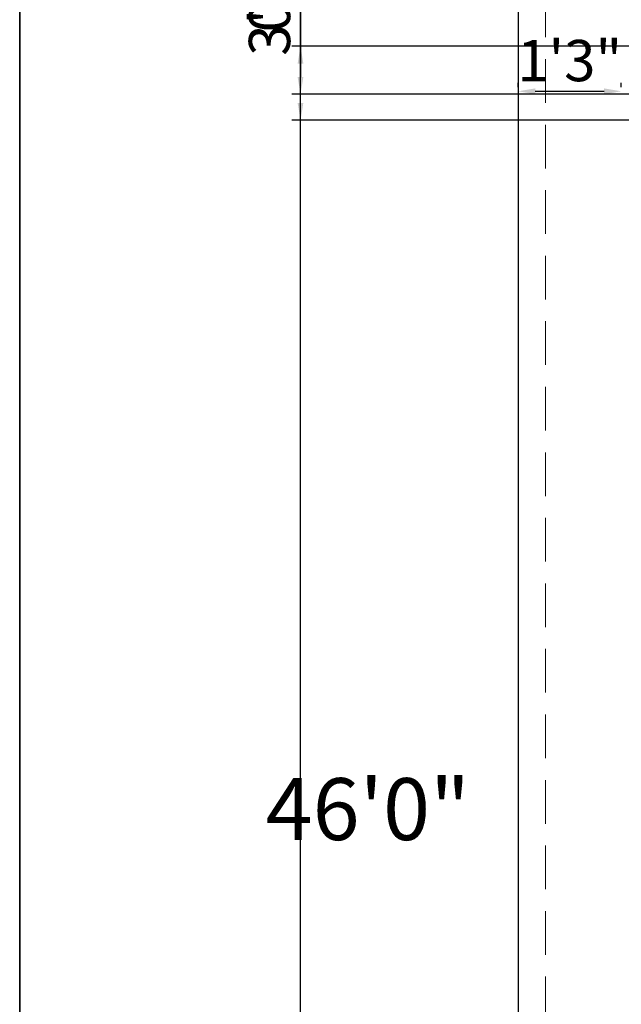
# Model space of a CAD drawing. Units: inches. Extents: x 2656 to 9931, y 1941 to 3068.
# Tile 4 of 46: x 2656 to 2743, y 2426 to 2569. Entities that reach past the tile are written whole.
import ezdxf

# ---------------------------------------------------------------- set-up
doc = ezdxf.new("R2010")
doc.units = ezdxf.units.IN
doc.linetypes.add('DASHED2', pattern=[9.525, 6.35, -3.175])
for name, color, linetype, lineweight in [('A-ANNO-DIMS', 2, 'Continuous', 18), ('A-ANNO-TTLB', 7, 'Continuous', 35), ('A-FLOR-OVHD', 252, 'DASHED2', 13), ('C-PROP', 7, 'Continuous', 25)]:
    doc.layers.add(name, color=color, linetype=linetype, lineweight=lineweight)
doc.styles.get("Standard").update_dxf_attribs({"font": 'arial.ttf'})
doc.dimstyles.new('ISO-25', dxfattribs={"dimtxt": 6, "dimasz": 2.5, "dimexe": 1.25, "dimexo": 0.625, "dimtad": 1, "dimdec": 0, "dimlunit": 3, "dimtxsty": 'Standard', "dimcen": 2.5, "dimadec": 0, "dimazin": 0, "dimtfac": 1, "dimtdec": 0, "dimtmove": 0, "dimatfit": 3, "dimfxl": 1, "dimarcsym": 0})

# ---------------------------------------------------------------- blocks, each defined once
blk = doc.blocks.new('*D1')
at = {"layer": 'A-ANNO-DIMS', "color": 0, "lineweight": -2, "transparency": 16777216}
for p, q in [((2728.16, 2559.42), (2728.16, 2560.05)), ((2730.66, 2558.8), (2740.66, 2558.8)), ((2743.16, 2559.42), (2743.16, 2560.05))]:
    blk.add_line(p, q, dxfattribs=at)
at = {"layer": 'A-ANNO-DIMS', "color": 0, "transparency": 16777216}
for points in [[(2730.66, 2559.22), (2730.66, 2558.38), (2728.16, 2558.8)], [(2740.66, 2559.22), (2740.66, 2558.38), (2743.16, 2558.8)]]:
    blk.add_solid(points, dxfattribs=at)
at = {"layer": 'Defpoints', "color": 0, "transparency": 16777216}
for p in [(2728.16, 2558.8), (2743.16, 2558.8), (2743.16, 2558.8)]:
    blk.add_point(p, dxfattribs=at)
at = {"layer": 'A-ANNO-DIMS', "color": 0, "transparency": 16777216, "insert": (2735.66, 2562.49), "char_height": 6, "attachment_point": 5}
blk.add_mtext('1\'3"', dxfattribs=at)
blk = doc.blocks.new('*D100')
at = {"layer": 'A-ANNO-DIMS', "color": 0, "lineweight": -2, "transparency": 16777216}
for p, q in [((2696.56, 2565.34), (2696.56, 2603.68)), ((2876.03, 2565.34), (2695.31, 2565.34)), ((2696.56, 2557.1), (2696.56, 2562.84)), ((2876.03, 2554.6), (2695.31, 2554.6))]:
    blk.add_line(p, q, dxfattribs=at)
at = {"layer": 'A-ANNO-DIMS', "color": 0, "transparency": 16777216}
for points in [[(2696.14, 2562.84), (2696.97, 2562.84), (2696.56, 2565.34)], [(2696.14, 2557.1), (2696.97, 2557.1), (2696.56, 2554.6)]]:
    blk.add_solid(points, dxfattribs=at)
at = {"layer": 'Defpoints', "color": 0, "transparency": 16777216}
for p in [(2696.56, 2565.34), (2876.66, 2565.34), (2876.66, 2554.6)]:
    blk.add_point(p, dxfattribs=at)
at = {"layer": 'A-ANNO-DIMS', "color": 0, "transparency": 16777216, "insert": (2692.83, 2585.76), "char_height": 6, "attachment_point": 5, "rotation": 90}
blk.add_mtext('0\'-10 1/2"', dxfattribs=at)
blk = doc.blocks.new('*D128')
at = {"layer": 'A-ANNO-DIMS', "color": 0, "lineweight": -2, "transparency": 16777216}
for p, q in [((2751.53, 2601.77), (2695.31, 2601.77)), ((2696.56, 2599.27), (2696.56, 2560.87)), ((2776.96, 2558.37), (2695.31, 2558.37))]:
    blk.add_line(p, q, dxfattribs=at)
at = {"layer": 'A-ANNO-DIMS', "color": 0, "transparency": 16777216}
for points in [[(2696.14, 2599.27), (2696.97, 2599.27), (2696.56, 2601.77)], [(2696.14, 2560.87), (2696.97, 2560.87), (2696.56, 2558.37)]]:
    blk.add_solid(points, dxfattribs=at)
at = {"layer": 'Defpoints', "color": 0, "transparency": 16777216}
for p in [(2752.16, 2601.77), (2696.56, 2558.37), (2777.59, 2558.37)]:
    blk.add_point(p, dxfattribs=at)
at = {"layer": 'A-ANNO-DIMS', "color": 0, "transparency": 16777216, "insert": (2692.83, 2580.07), "char_height": 6, "attachment_point": 5, "rotation": 90}
blk.add_mtext('3\'-7 1/2"', dxfattribs=at)
blk = doc.blocks.new('*D175')
at = {"layer": 'A-ANNO-DIMS', "color": 0, "lineweight": -2, "transparency": 16777216}
for p, q in [((2742.53, 2623.6), (2695.31, 2623.6)), ((2696.56, 2169.1), (2696.56, 2621.1)), ((2742.53, 2166.6), (2695.31, 2166.6))]:
    blk.add_line(p, q, dxfattribs=at)
at = {"layer": 'A-ANNO-DIMS', "color": 0, "transparency": 16777216}
for points in [[(2696.14, 2621.1), (2696.97, 2621.1), (2696.56, 2623.6)], [(2696.14, 2169.1), (2696.97, 2169.1), (2696.56, 2166.6)]]:
    blk.add_solid(points, dxfattribs=at)
at = {"layer": 'Defpoints', "color": 0, "transparency": 16777216}
for p in [(2696.56, 2623.6), (2743.16, 2623.6), (2743.16, 2166.6)]:
    blk.add_point(p, dxfattribs=at)
at = {"layer": 'A-ANNO-DIMS', "color": 0, "transparency": 16777216, "insert": (2692.87, 2395.1), "char_height": 6, "attachment_point": 5, "rotation": 90}
blk.add_mtext('38\'-1"', dxfattribs=at)

msp = doc.modelspace()

# ---------------------------------------------------------------- linework, layer by layer
at = {"layer": 'A-ANNO-TTLB'}
msp.add_lwpolyline([(2655.77, 3067.84), (3515.43, 3067.84), (3515.43, 1940.89), (2655.77, 1940.89)], close=True, dxfattribs=at)
at = {"layer": 'A-FLOR-OVHD'}
msp.add_line((2732.16, 2166.6), (2732.16, 2637.6), dxfattribs=at)
at = {"layer": 'C-PROP'}
msp.add_line((2728.16, 2641.6), (2728.16, 2086.1), dxfattribs=at)

# ---------------------------------------------------------------- texts
at = {"layer": 'A-ANNO-DIMS', "insert": (2691.51, 2458.97), "char_height": 9, "attachment_point": 1}
msp.add_mtext_dynamic_manual_height_columns('46\'0"', width=227.8952, gutter_width=12.5, heights=[0], dxfattribs=at)

# ---------------------------------------------------------------- dimensions: what is measured, and where the dimension line sits
at = {"layer": 'A-ANNO-DIMS'}
for base, p1, p2, picture, middle in [((2696.56, 2623.6), (2743.16, 2166.6), (2743.16, 2623.6), '*D175', (2692.87, 2395.1)), ((2696.56, 2565.34), (2876.66, 2554.6), (2876.66, 2565.34), '*D100', (2692.83, 2585.76)), ((2696.56, 2558.37), (2752.16, 2601.77), (2777.59, 2558.37), '*D128', (2692.83, 2580.07))]:
    dim = msp.add_linear_dim(base=base, p1=p1, p2=p2, angle=90, dimstyle='ISO-25', override={"dimdec": 1, "dimlfac": 1, "dimrnd": 0, "dimzin": 1, "dimdsep": 46, "dimlunit": 4, "dimfrac": 2}, dxfattribs=at)
    dim.commit()
    dim.dimension.update_dxf_attribs({"geometry": picture, "text_midpoint": middle})
dim = msp.add_linear_dim(base=(2743.16, 2558.8), p1=(2728.16, 2558.8), p2=(2743.16, 2558.8), text='1\'3"', dimstyle='ISO-25', override={"dimclrd": 0, "dimclre": 0, "dimclrt": 0}, dxfattribs=at)
dim.commit()
dim.dimension.update_dxf_attribs({"geometry": '*D1', "text_midpoint": (2735.66, 2562.49)})

doc.saveas('drawing.dxf')
